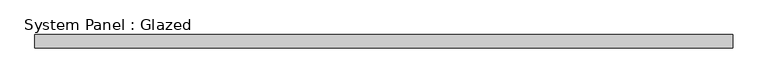
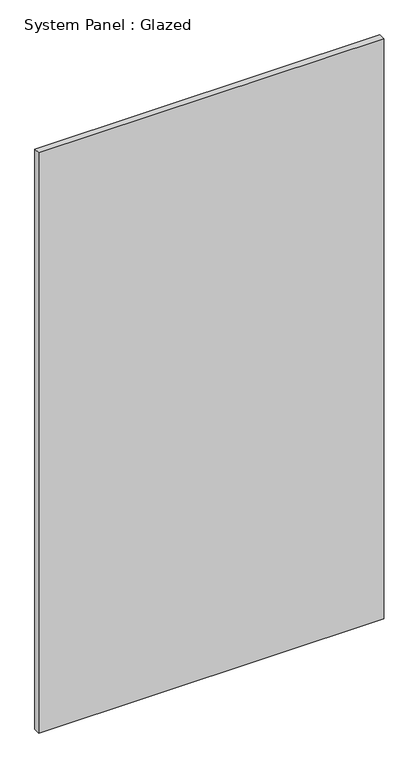
"""IFC4 building model written with IfcOpenShell, lengths in millimetres: plate geometry, System Panel : Glazed."""

from ifc_helpers import new_model, si_unit, origin, origin_with_axes, place, context, project, spatial, polyline, outline, extrude, source, transform, mapped, element, save


def system_panel_glazed_e2c3efe7(model_context):
    return source(origin(), model_context, "Body", "SweptSolid", [
        extrude(outline(polyline([(667.8083334, 19.05), (-667.8083334, 19.05), (-667.8083334, 44.45), (667.8083334, 44.45), (667.8083334, 19.05)])), origin_with_axes(), (0.0, 0.0, 1.0), 2374.9),
    ])


if __name__ == "__main__":
    model = new_model("IFC4")
    model_context = context("Model", 3, world=origin())
    ifc_project = project(units=[si_unit("LENGTHUNIT", "METRE", prefix="MILLI")], contexts=[model_context])
    site = spatial("IfcSite", under=ifc_project)
    building = spatial("IfcBuilding", under=site)
    placement = place(None, origin())
    system_panel_glazed_shape = system_panel_glazed_e2c3efe7(model_context)
    element("IfcPlate", 1, ObjectType="System Panel : Glazed", at=placement, inside=building, context=model_context, shape_type="MappedRepresentation", body=[
        mapped(system_panel_glazed_shape, transform((0.0, 0.0, 0.0), x_axis=(1.0, 0.0, 0.0), y_axis=(0.0, 1.0, 0.0), z_axis=(0.0, 0.0, 1.0))),
    ])
    save(model, "model.ifc")

# Revit data of these elements
# Type "System Panel : Glazed"
#   Construction Type Id = "GSP4R"
#   Analytic Construction = "1/8 in Pilkington single glazing"
#   Visual Light Transmittance = 0.9
#   Solar Heat Gain Coefficient = 0.86
#   Heat Transfer Coefficient (U) = 1.18115 BTU/(h·ft²·°F)
#   Define Thermal Properties by = 1
# Element 1 (IfcPlate, "System Panel : Glazed")
#   Materials on its faces: "Glass"
# Materials
#   "Glass": class "Glass", colour RGB 0 128 192, transparency 0.75, Description = "Soda Lime Glass", Cost = 0
